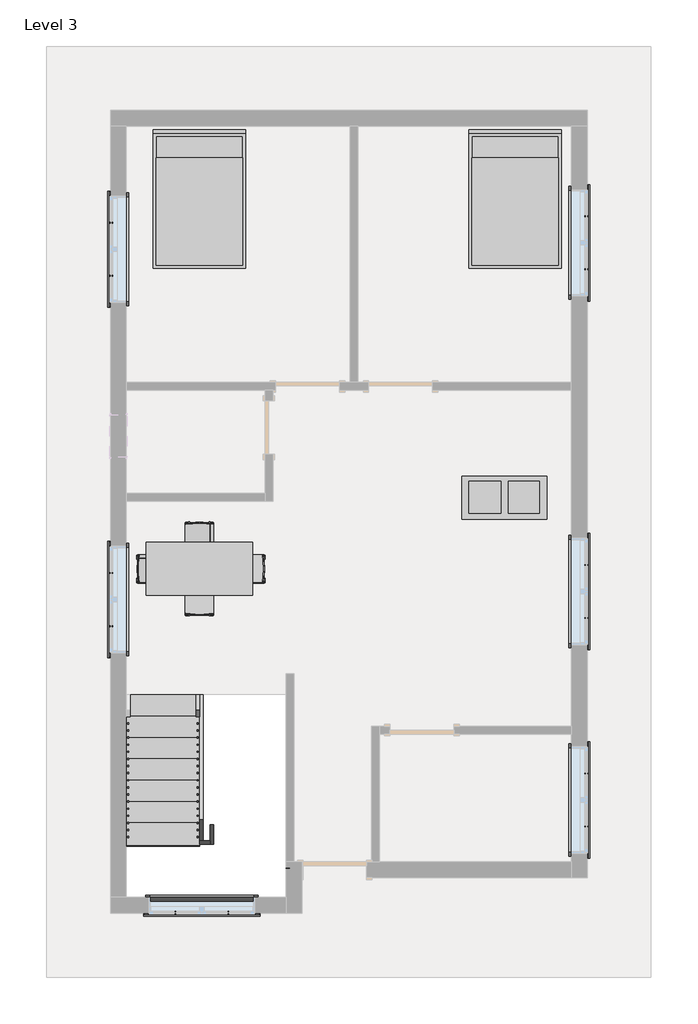
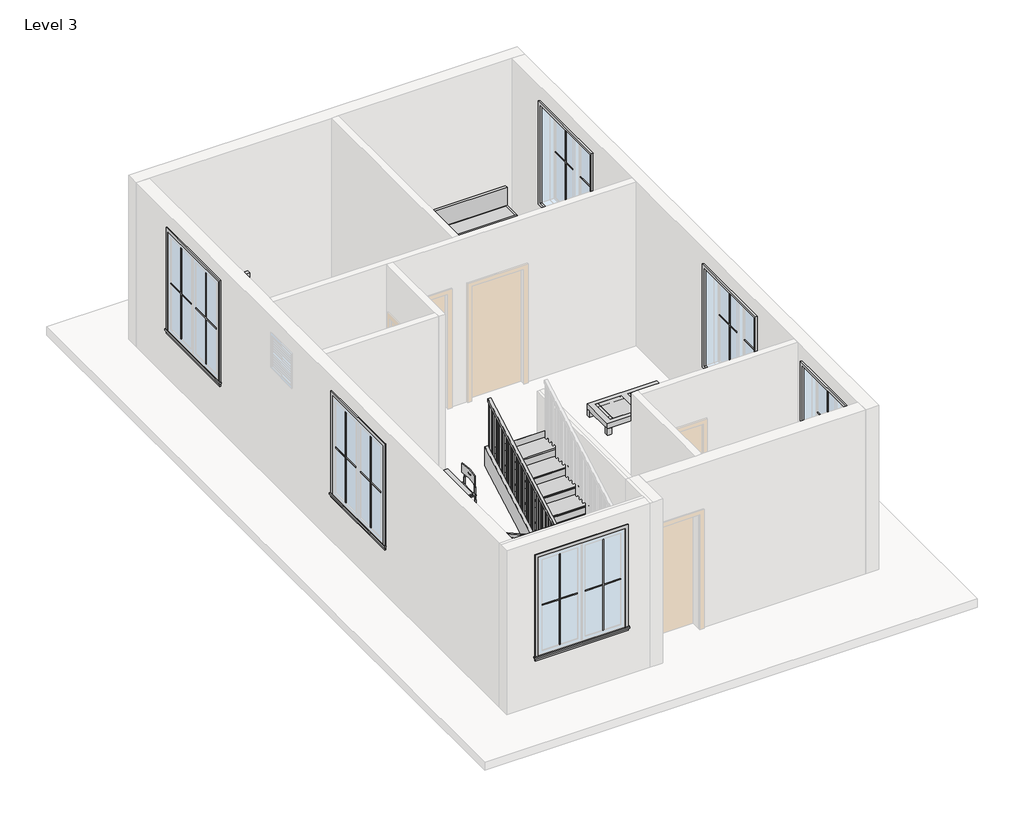
# One storey, part 3 of 3: 25 proxies, 6 members, 3 furniture elements, 1 railing, 1 stair flight.
"""IFC4 building model written with IfcOpenShell, lengths in millimetres."""

from ifc_helpers import new_model, si_unit, frame, origin, place, context, project, spatial, polyline, outline, extrude, faceted_brep, transform, mapped, element, save
from components import muntin_pattern_2x2_muntin_pattern_2x2_f6a80940, muntin_pattern_2x2_muntin_pattern_2x2_09b00a1c, trim_window_exterior_flat_with_sill_698ed857, trim_window_interior_flat_picture_frame_92551a5e, coffee_table_with_brass_mullions_11320_coffee_table_with_5962bef7, bed_17739_bed_17739_15c61121, dining_table_w_chairs_11374_0cdfc61b, stair_flight_c3010b6b

model = new_model("IFC4")

# Units and contexts
model_context = context("Model", 3, world=origin())
ifc_project = project(units=[si_unit("LENGTHUNIT", "METRE", prefix="MILLI")], contexts=[model_context])

# Site, building, storey
site = spatial("IfcSite", under=ifc_project)
building = spatial("IfcBuilding", under=site)
storey = spatial("IfcBuildingStorey", under=building, Name="Level 3", Elevation=6248.4)

# Proxies
placement = place(None, origin())
muntin_pattern_2x2_muntin_pattern_2x2_shape = muntin_pattern_2x2_muntin_pattern_2x2_f6a80940(model_context)
element("IfcBuildingElementProxy", 1, Name="Muntin Pattern_2x2 : Muntin Pattern_2x2", ObjectType="Muntin Pattern_2x2 : Muntin Pattern_2x2", at=placement, inside=storey, context=model_context, shape_type="MappedRepresentation", body=[
    mapped(muntin_pattern_2x2_muntin_pattern_2x2_shape, transform((-2773.368364, -6686.2830018, 7232.65), x_axis=(-1.0, 0.0, 0.0), y_axis=(0.0, -1.0, 0.0), z_axis=(0.0, 0.0, 1.0))),
])
element("IfcBuildingElementProxy", 2, Name="Muntin Pattern_2x2 : Muntin Pattern_2x2", ObjectType="Muntin Pattern_2x2 : Muntin Pattern_2x2", at=placement, inside=storey, context=model_context, shape_type="MappedRepresentation", body=[
    mapped(muntin_pattern_2x2_muntin_pattern_2x2_shape, transform((2349.494136, -4693.9705018, 7232.65), x_axis=(0.0, -1.0, 0.0), y_axis=(1.0, 0.0, 0.0), z_axis=(0.0, 0.0, 1.0))),
])
element("IfcBuildingElementProxy", 3, Name="Muntin Pattern_2x2 : Muntin Pattern_2x2", ObjectType="Muntin Pattern_2x2 : Muntin Pattern_2x2", at=placement, inside=storey, context=model_context, shape_type="MappedRepresentation", body=[
    mapped(muntin_pattern_2x2_muntin_pattern_2x2_shape, transform((2349.494136, -1712.6455018, 7232.65), x_axis=(0.0, -1.0, 0.0), y_axis=(1.0, 0.0, 0.0), z_axis=(0.0, 0.0, 1.0))),
])
element("IfcBuildingElementProxy", 4, Name="Muntin Pattern_2x2 : Muntin Pattern_2x2", ObjectType="Muntin Pattern_2x2 : Muntin Pattern_2x2", at=placement, inside=storey, context=model_context, shape_type="MappedRepresentation", body=[
    mapped(muntin_pattern_2x2_muntin_pattern_2x2_shape, transform((-4451.355864, -2586.5525081, 7232.65), x_axis=(0.0, 1.0, 0.0), y_axis=(-1.0, 0.0, 0.0), z_axis=(0.0, 0.0, 1.0))),
])
element("IfcBuildingElementProxy", 5, Name="Muntin Pattern_2x2 : Muntin Pattern_2x2", ObjectType="Muntin Pattern_2x2 : Muntin Pattern_2x2", at=placement, inside=storey, context=model_context, shape_type="MappedRepresentation", body=[
    mapped(muntin_pattern_2x2_muntin_pattern_2x2_shape, transform((2349.494136, 3272.1044982, 7232.65), x_axis=(0.0, -1.0, 0.0), y_axis=(1.0, 0.0, 0.0), z_axis=(0.0, 0.0, 1.0))),
])
element("IfcBuildingElementProxy", 6, Name="Muntin Pattern_2x2 : Muntin Pattern_2x2", ObjectType="Muntin Pattern_2x2 : Muntin Pattern_2x2", at=placement, inside=storey, context=model_context, shape_type="MappedRepresentation", body=[
    mapped(muntin_pattern_2x2_muntin_pattern_2x2_shape, transform((-4451.355864, 2421.2162133, 7232.65), x_axis=(0.0, 1.0, 0.0), y_axis=(-1.0, 0.0, 0.0), z_axis=(0.0, 0.0, 1.0))),
])
muntin_pattern_2x2_muntin_pattern_2x2_2_shape = muntin_pattern_2x2_muntin_pattern_2x2_09b00a1c(model_context)
element("IfcBuildingElementProxy", 7, Name="Muntin Pattern_2x2 : Muntin Pattern_2x2", ObjectType="Muntin Pattern_2x2 : Muntin Pattern_2x2", at=placement, inside=storey, context=model_context, shape_type="MappedRepresentation", body=[
    mapped(muntin_pattern_2x2_muntin_pattern_2x2_2_shape, transform((-3532.193364, -6686.2830018, 7232.65), x_axis=(1.0, 0.0, 0.0), y_axis=(0.0, 1.0, 0.0), z_axis=(0.0, 0.0, 1.0))),
])
element("IfcBuildingElementProxy", 8, Name="Muntin Pattern_2x2 : Muntin Pattern_2x2", ObjectType="Muntin Pattern_2x2 : Muntin Pattern_2x2", at=placement, inside=storey, context=model_context, shape_type="MappedRepresentation", body=[
    mapped(muntin_pattern_2x2_muntin_pattern_2x2_2_shape, transform((2349.494136, -5452.7955018, 7232.65), x_axis=(0.0, 1.0, 0.0), y_axis=(-1.0, 0.0, 0.0), z_axis=(0.0, 0.0, 1.0))),
])
element("IfcBuildingElementProxy", 9, Name="Muntin Pattern_2x2 : Muntin Pattern_2x2", ObjectType="Muntin Pattern_2x2 : Muntin Pattern_2x2", at=placement, inside=storey, context=model_context, shape_type="MappedRepresentation", body=[
    mapped(muntin_pattern_2x2_muntin_pattern_2x2_2_shape, transform((2349.494136, -2471.4705018, 7232.65), x_axis=(0.0, 1.0, 0.0), y_axis=(-1.0, 0.0, 0.0), z_axis=(0.0, 0.0, 1.0))),
])
element("IfcBuildingElementProxy", 10, Name="Muntin Pattern_2x2 : Muntin Pattern_2x2", ObjectType="Muntin Pattern_2x2 : Muntin Pattern_2x2", at=placement, inside=storey, context=model_context, shape_type="MappedRepresentation", body=[
    mapped(muntin_pattern_2x2_muntin_pattern_2x2_2_shape, transform((-4451.355864, -1827.7275081, 7232.65), x_axis=(0.0, -1.0, 0.0), y_axis=(1.0, 0.0, 0.0), z_axis=(0.0, 0.0, 1.0))),
])
element("IfcBuildingElementProxy", 11, Name="Muntin Pattern_2x2 : Muntin Pattern_2x2", ObjectType="Muntin Pattern_2x2 : Muntin Pattern_2x2", at=placement, inside=storey, context=model_context, shape_type="MappedRepresentation", body=[
    mapped(muntin_pattern_2x2_muntin_pattern_2x2_2_shape, transform((2349.494136, 2513.2794982, 7232.65), x_axis=(0.0, 1.0, 0.0), y_axis=(-1.0, 0.0, 0.0), z_axis=(0.0, 0.0, 1.0))),
])
element("IfcBuildingElementProxy", 12, Name="Muntin Pattern_2x2 : Muntin Pattern_2x2", ObjectType="Muntin Pattern_2x2 : Muntin Pattern_2x2", at=placement, inside=storey, context=model_context, shape_type="MappedRepresentation", body=[
    mapped(muntin_pattern_2x2_muntin_pattern_2x2_2_shape, transform((-4451.355864, 3180.0412133, 7232.65), x_axis=(0.0, -1.0, 0.0), y_axis=(1.0, 0.0, 0.0), z_axis=(0.0, 0.0, 1.0))),
])
trim_window_exterior_flat_with_sill_shape = trim_window_exterior_flat_with_sill_698ed857(model_context)
element("IfcBuildingElementProxy", 13, Name="Trim-Window-Exterior-Flat : with Sill", ObjectType="Trim-Window-Exterior-Flat : with Sill", at=placement, inside=storey, context=model_context, shape_type="MappedRepresentation", body=[
    mapped(trim_window_exterior_flat_with_sill_shape, transform((-3152.780864, -6695.8080018, 8991.6), x_axis=(1.0, 0.0, 0.0), y_axis=(0.0, 0.0, 1.0), z_axis=(0.0, -1.0, 0.0))),
])
element("IfcBuildingElementProxy", 14, Name="Trim-Window-Exterior-Flat : with Sill", ObjectType="Trim-Window-Exterior-Flat : with Sill", at=placement, inside=storey, context=model_context, shape_type="MappedRepresentation", body=[
    mapped(trim_window_exterior_flat_with_sill_shape, transform((2359.019136, -5073.3830018, 8991.6), x_axis=(0.0, 1.0, 0.0), y_axis=(0.0, 0.0, 1.0), z_axis=(1.0, 0.0, 0.0))),
])
element("IfcBuildingElementProxy", 15, Name="Trim-Window-Exterior-Flat : with Sill", ObjectType="Trim-Window-Exterior-Flat : with Sill", at=placement, inside=storey, context=model_context, shape_type="MappedRepresentation", body=[
    mapped(trim_window_exterior_flat_with_sill_shape, transform((2359.019136, -2092.0580018, 8991.6), x_axis=(0.0, 1.0, 0.0), y_axis=(0.0, 0.0, 1.0), z_axis=(1.0, 0.0, 0.0))),
])
element("IfcBuildingElementProxy", 16, Name="Trim-Window-Exterior-Flat : with Sill", ObjectType="Trim-Window-Exterior-Flat : with Sill", at=placement, inside=storey, context=model_context, shape_type="MappedRepresentation", body=[
    mapped(trim_window_exterior_flat_with_sill_shape, transform((-4460.880864, -2207.1400081, 8991.6), x_axis=(0.0, -1.0, 0.0), y_axis=(0.0, 0.0, 1.0), z_axis=(-1.0, 0.0, 0.0))),
])
element("IfcBuildingElementProxy", 17, Name="Trim-Window-Exterior-Flat : with Sill", ObjectType="Trim-Window-Exterior-Flat : with Sill", at=placement, inside=storey, context=model_context, shape_type="MappedRepresentation", body=[
    mapped(trim_window_exterior_flat_with_sill_shape, transform((2359.019136, 2892.6919982, 8991.6), x_axis=(0.0, 1.0, 0.0), y_axis=(0.0, 0.0, 1.0), z_axis=(1.0, 0.0, 0.0))),
])
element("IfcBuildingElementProxy", 18, Name="Trim-Window-Exterior-Flat : with Sill", ObjectType="Trim-Window-Exterior-Flat : with Sill", at=placement, inside=storey, context=model_context, shape_type="MappedRepresentation", body=[
    mapped(trim_window_exterior_flat_with_sill_shape, transform((-4460.880864, 2800.6287133, 8991.6), x_axis=(0.0, -1.0, 0.0), y_axis=(0.0, 0.0, 1.0), z_axis=(-1.0, 0.0, 0.0))),
])
trim_window_interior_flat_picture_frame_shape = trim_window_interior_flat_picture_frame_92551a5e(model_context)
element("IfcBuildingElementProxy", 19, Name="Trim-Window-Interior-Flat : Picture Frame", ObjectType="Trim-Window-Interior-Flat : Picture Frame", at=placement, inside=storey, context=model_context, shape_type="MappedRepresentation", body=[
    mapped(trim_window_interior_flat_picture_frame_shape, transform((-3152.780864, -6467.2080018, 8991.6), x_axis=(-1.0, 0.0, 0.0), y_axis=(0.0, 0.0, 1.0), z_axis=(0.0, 1.0, 0.0))),
])
element("IfcBuildingElementProxy", 20, Name="Trim-Window-Interior-Flat : Picture Frame", ObjectType="Trim-Window-Interior-Flat : Picture Frame", at=placement, inside=storey, context=model_context, shape_type="MappedRepresentation", body=[
    mapped(trim_window_interior_flat_picture_frame_shape, transform((2130.419136, -5073.3830018, 8991.6), x_axis=(0.0, -1.0, 0.0), y_axis=(0.0, 0.0, 1.0), z_axis=(-1.0, 0.0, 0.0))),
])
element("IfcBuildingElementProxy", 21, Name="Trim-Window-Interior-Flat : Picture Frame", ObjectType="Trim-Window-Interior-Flat : Picture Frame", at=placement, inside=storey, context=model_context, shape_type="MappedRepresentation", body=[
    mapped(trim_window_interior_flat_picture_frame_shape, transform((2130.419136, -2092.0580018, 8991.6), x_axis=(0.0, -1.0, 0.0), y_axis=(0.0, 0.0, 1.0), z_axis=(-1.0, 0.0, 0.0))),
])
element("IfcBuildingElementProxy", 22, Name="Trim-Window-Interior-Flat : Picture Frame", ObjectType="Trim-Window-Interior-Flat : Picture Frame", at=placement, inside=storey, context=model_context, shape_type="MappedRepresentation", body=[
    mapped(trim_window_interior_flat_picture_frame_shape, transform((-4232.280864, -2207.1400081, 8991.6), x_axis=(0.0, 1.0, 0.0), y_axis=(0.0, 0.0, 1.0), z_axis=(1.0, 0.0, 0.0))),
])
element("IfcBuildingElementProxy", 23, Name="Trim-Window-Interior-Flat : Picture Frame", ObjectType="Trim-Window-Interior-Flat : Picture Frame", at=placement, inside=storey, context=model_context, shape_type="MappedRepresentation", body=[
    mapped(trim_window_interior_flat_picture_frame_shape, transform((2130.419136, 2892.6919982, 8991.6), x_axis=(0.0, -1.0, 0.0), y_axis=(0.0, 0.0, 1.0), z_axis=(-1.0, 0.0, 0.0))),
])
element("IfcBuildingElementProxy", 24, Name="Trim-Window-Interior-Flat : Picture Frame", ObjectType="Trim-Window-Interior-Flat : Picture Frame", at=placement, inside=storey, context=model_context, shape_type="MappedRepresentation", body=[
    mapped(trim_window_interior_flat_picture_frame_shape, transform((-4232.280864, 2800.6287133, 8991.6), x_axis=(0.0, 1.0, 0.0), y_axis=(0.0, 0.0, 1.0), z_axis=(1.0, 0.0, 0.0))),
])
coffee_table_with_brass_mullions_11320_coffee_table_with_shape = coffee_table_with_brass_mullions_11320_coffee_table_with_5962bef7(model_context)
element("IfcBuildingElementProxy", 25, Name="coffee_table_with_brass_mullions_11320 : coffee_table_with_brass_mullions_11320", ObjectType="coffee_table_with_brass_mullions_11320 : coffee_table_with_brass_mullions_11320", at=placement, inside=storey, context=model_context, shape_type="MappedRepresentation", body=[
    mapped(coffee_table_with_brass_mullions_11320_coffee_table_with_shape, transform((1812.3816081, -1181.1001099, 6248.4), x_axis=(1.0, 0.0, 0.0), y_axis=(0.0, 1.0, 0.0), z_axis=(0.0, 0.0, 1.0))),
])

# Furniture
bed_17739_bed_17739_shape = bed_17739_bed_17739_15c61121(model_context)
element("IfcFurniture", 26, ObjectType="Bed_17739 : Bed_17739", at=placement, inside=storey, context=model_context, shape_type="MappedRepresentation", body=[
    mapped(bed_17739_bed_17739_shape, transform((1328.5116081, 3496.3098901, 6248.4), x_axis=(1.0, 0.0, 0.0), y_axis=(0.0, 1.0, 0.0), z_axis=(0.0, 0.0, 1.0))),
])
element("IfcFurniture", 27, ObjectType="Bed_17739 : Bed_17739", at=placement, inside=storey, context=model_context, shape_type="MappedRepresentation", body=[
    mapped(bed_17739_bed_17739_shape, transform((-3187.6083919, 3496.3098901, 6248.4), x_axis=(1.0, 0.0, 0.0), y_axis=(0.0, 1.0, 0.0), z_axis=(0.0, 0.0, 1.0))),
])
dining_table_w_chairs_11374_shape = dining_table_w_chairs_11374_0cdfc61b(model_context)
element("IfcFurniture", 28, ObjectType="Dining_Table_w_Chairs_11374", at=placement, inside=storey, context=model_context, shape_type="MappedRepresentation", body=[
    mapped(dining_table_w_chairs_11374_shape, transform((-3205.8741586, -1863.0511877, 6248.4), x_axis=(1.0, 0.0, 0.0), y_axis=(0.0, 1.0, 0.0), z_axis=(0.0, 0.0, 1.0))),
])

# Members
element("IfcMember", 29, ObjectType="Stringer - 2\" Width", at=placement, inside=storey, context=model_context, shape_type="SweptSolid", body=[
    extrude(outline(polyline([(-3571.6080018, 6455.9983948), (-3571.6080018, 6248.4), (-3825.5525046, 6248.4), (-5654.4080018, 7264.4308318), (-5654.4080018, 7613.1095059), (-3571.6080018, 6455.9983948)])), frame((-3187.6083919, 0.0, 0.0), z_axis=(1.0, 0.0, 0.0), x_axis=(0.0, 1.0, 0.0)), (0.0, 0.0, 1.0), 50.8),
])
element("IfcMember", 30, ObjectType="Stringer - 2\" Width", at=placement, inside=storey, context=model_context, shape_type="SweptSolid", body=[
    extrude(outline(polyline([(-3187.6083919, -5705.2080018), (-3187.6083919, -5654.4080018), (-3035.2083919, -5654.4080018), (-3035.2083919, -5705.2080018), (-3187.6083919, -5705.2080018)])), frame((0.0, 0.0, 7374.4666667), z_axis=(0.0, 0.0, 1.0), x_axis=(1.0, 0.0, 0.0)), (0.0, 0.0, 1.0), 304.8),
])
element("IfcMember", 31, ObjectType="Stringer - 2\" Width", at=placement, inside=storey, context=model_context, shape_type="SweptSolid", body=[
    extrude(outline(polyline([(-5705.2080018, 7374.4666667), (-5705.2080018, 7641.3317281), (-3571.6080018, 8826.6650614), (-3571.6080018, 8477.9863873), (-5557.943499, 7374.4666667), (-5705.2080018, 7374.4666667)])), frame((-3035.2083919, 0.0, 0.0), z_axis=(1.0, 0.0, 0.0), x_axis=(0.0, 1.0, 0.0)), (0.0, 0.0, 1.0), 50.8),
])
element("IfcMember", 32, ObjectType="Stringer - 2\" Width", at=placement, inside=storey, context=model_context, shape_type="SweptSolid", body=[
    extrude(outline(polyline([(-3571.6080018, 6455.9983948), (-3571.6080018, 6248.4), (-3825.5525046, 6248.4), (-6401.1125046, 7679.2666667), (-5773.4908912, 7679.2666667), (-3571.6080018, 6455.9983948)])), frame((-4283.080864, 0.0, 0.0), z_axis=(1.0, 0.0, 0.0), x_axis=(0.0, 1.0, 0.0)), (0.0, 0.0, 1.0), 50.8),
])
element("IfcMember", 33, ObjectType="Stringer - 2\" Width", at=placement, inside=storey, context=model_context, shape_type="SweptSolid", body=[
    extrude(outline(polyline([(-4283.080864, -6518.0080018), (-4283.080864, -6467.2080018), (-1946.280864, -6467.2080018), (-1946.280864, -6518.0080018), (-4283.080864, -6518.0080018)])), frame((0.0, 0.0, 7374.4666667), z_axis=(0.0, 0.0, 1.0), x_axis=(1.0, 0.0, 0.0)), (0.0, 0.0, 1.0), 304.8),
])
element("IfcMember", 34, ObjectType="Stringer - 2\" Width", at=placement, inside=storey, context=model_context, shape_type="SweptSolid", body=[
    extrude(outline(polyline([(-6185.5651124, 7374.4666667), (-3571.6080018, 8826.6650614), (-3571.6080018, 8477.9863873), (-5557.943499, 7374.4666667), (-6185.5651124, 7374.4666667)])), frame((-1946.280864, 0.0, 0.0), z_axis=(1.0, 0.0, 0.0), x_axis=(0.0, 1.0, 0.0)), (0.0, 0.0, 1.0), 50.8),
])

# Railing
element("IfcRailing", 35, ObjectType="Handrail - Rectangular", at=placement, inside=storey, context=model_context, shape_type="SolidModel", body=[
    faceted_brep([(-3187.6083919, -3571.6080018, 7332.1333333), (-3187.6083919, -3571.6080018, 7274.020221), (-3238.4083919, -3571.6080018, 7274.020221), (-3238.4083919, -3571.6080018, 7332.1333333), (-3187.6083919, -5629.0080018, 8475.1333333), (-3187.6083919, -5679.8080018, 8445.2424432), (-3238.4083919, -5679.8080018, 8445.2424432), (-3238.4083919, -5629.0080018, 8475.1333333), (-3187.6083919, -5629.0080018, 8517.4666667), (-3187.6083919, -5679.8080018, 8466.6666667), (-3238.4083919, -5679.8080018, 8466.6666667), (-3238.4083919, -5629.0080018, 8517.4666667), (-3187.6083919, -5705.2080018, 8517.4666667), (-3187.6083919, -5705.2080018, 8466.6666667), (-3238.4083919, -5756.0080018, 8466.6666667), (-3238.4083919, -5756.0080018, 8517.4666667), (-3111.4083919, -5705.2080018, 8517.4666667), (-3111.4083919, -5705.2080018, 8466.6666667), (-3111.4083919, -5756.0080018, 8466.6666667), (-3111.4083919, -5756.0080018, 8517.4666667), (-3060.6083919, -5705.2080018, 8517.4666667), (-3009.8083919, -5705.2080018, 8466.6666667), (-3009.8083919, -5756.0080018, 8466.6666667), (-3060.6083919, -5756.0080018, 8517.4666667), (-3060.6083919, -5705.2080018, 8559.8), (-3009.8083919, -5705.2080018, 8509.0), (-3009.8083919, -5756.0080018, 8509.0), (-3060.6083919, -5756.0080018, 8559.8), (-2984.4083919, -5705.2080018, 8559.8), (-2984.4083919, -5705.2080018, 8509.0), (-2933.6083919, -5756.0080018, 8509.0), (-2933.6083919, -5756.0080018, 8559.8), (-2984.4083919, -5629.0080018, 8559.8), (-2984.4083919, -5615.8443995, 8509.0), (-2933.6083919, -5615.8443995, 8509.0), (-2933.6083919, -5629.0080018, 8559.8), (-2984.4083919, -3571.6080018, 9702.8), (-2933.6083919, -3571.6080018, 9702.8), (-2933.6083919, -3571.6080018, 9644.6868876), (-2984.4083919, -3571.6080018, 9644.6868876)], [[[0, 1, 2, 3]], [[1, 0, 4, 5]], [[2, 1, 5, 6]], [[3, 2, 6, 7]], [[0, 3, 7, 4]], [[5, 4, 8, 9]], [[6, 5, 9, 10]], [[7, 6, 10, 11]], [[4, 7, 11, 8]], [[9, 8, 12, 13]], [[10, 9, 13, 14]], [[11, 10, 14, 15]], [[8, 11, 15, 12]], [[13, 12, 16, 17]], [[14, 13, 17, 18]], [[15, 14, 18, 19]], [[12, 15, 19, 16]], [[17, 16, 20, 21]], [[18, 17, 21, 22]], [[19, 18, 22, 23]], [[16, 19, 23, 20]], [[21, 20, 24, 25]], [[22, 21, 25, 26]], [[23, 22, 26, 27]], [[20, 23, 27, 24]], [[25, 24, 28, 29]], [[26, 25, 29, 30]], [[27, 26, 30, 31]], [[24, 27, 31, 28]], [[29, 28, 32, 33]], [[30, 29, 33, 34]], [[31, 30, 34, 35]], [[28, 31, 35, 32]], [[36, 37, 38, 39]], [[33, 32, 36, 39]], [[34, 33, 39, 38]], [[35, 34, 38, 37]], [[32, 35, 37, 36]]]),
    extrude(outline(polyline([(-3587.4830018, 9635.8674432), (-3587.4830018, 8619.0666667), (-3606.5330018, 8619.0666667), (-3606.5330018, 9625.2841099), (-3587.4830018, 9635.8674432)])), frame((-2968.5333919, 0.0, 0.0), z_axis=(1.0, 0.0, 0.0), x_axis=(0.0, 1.0, 0.0)), (0.0, 0.0, 1.0), 19.05),
    extrude(outline(polyline([(-3689.0830018, 9579.4229988), (-3689.0830018, 8619.0666667), (-3708.1330018, 8619.0666667), (-3708.1330018, 9568.8396654), (-3689.0830018, 9579.4229988)])), frame((-2968.5333919, 0.0, 0.0), z_axis=(1.0, 0.0, 0.0), x_axis=(0.0, 1.0, 0.0)), (0.0, 0.0, 1.0), 19.05),
    extrude(outline(polyline([(-3790.6830018, 9522.9785543), (-3790.6830018, 8619.0666667), (-3809.7330018, 8619.0666667), (-3809.7330018, 9512.395221), (-3790.6830018, 9522.9785543)])), frame((-2968.5333919, 0.0, 0.0), z_axis=(1.0, 0.0, 0.0), x_axis=(0.0, 1.0, 0.0)), (0.0, 0.0, 1.0), 19.05),
    extrude(outline(polyline([(-3892.2830018, 9466.5341099), (-3892.2830018, 8449.7333333), (-3911.3330018, 8449.7333333), (-3911.3330018, 9455.9507765), (-3892.2830018, 9466.5341099)])), frame((-2968.5333919, 0.0, 0.0), z_axis=(1.0, 0.0, 0.0), x_axis=(0.0, 1.0, 0.0)), (0.0, 0.0, 1.0), 19.05),
    extrude(outline(polyline([(-3993.8830018, 9410.0896654), (-3993.8830018, 8449.7333333), (-4012.9330018, 8449.7333333), (-4012.9330018, 9399.5063321), (-3993.8830018, 9410.0896654)])), frame((-2968.5333919, 0.0, 0.0), z_axis=(1.0, 0.0, 0.0), x_axis=(0.0, 1.0, 0.0)), (0.0, 0.0, 1.0), 19.05),
    extrude(outline(polyline([(-4095.4830018, 9353.645221), (-4095.4830018, 8449.7333333), (-4114.5330018, 8449.7333333), (-4114.5330018, 9343.0618876), (-4095.4830018, 9353.645221)])), frame((-2968.5333919, 0.0, 0.0), z_axis=(1.0, 0.0, 0.0), x_axis=(0.0, 1.0, 0.0)), (0.0, 0.0, 1.0), 19.05),
    extrude(outline(polyline([(-4197.0830018, 9297.2007765), (-4197.0830018, 8280.4), (-4216.1330018, 8280.4), (-4216.1330018, 9286.6174432), (-4197.0830018, 9297.2007765)])), frame((-2968.5333919, 0.0, 0.0), z_axis=(1.0, 0.0, 0.0), x_axis=(0.0, 1.0, 0.0)), (0.0, 0.0, 1.0), 19.05),
    extrude(outline(polyline([(-4298.6830018, 9240.7563321), (-4298.6830018, 8280.4), (-4317.7330018, 8280.4), (-4317.7330018, 9230.1729988), (-4298.6830018, 9240.7563321)])), frame((-2968.5333919, 0.0, 0.0), z_axis=(1.0, 0.0, 0.0), x_axis=(0.0, 1.0, 0.0)), (0.0, 0.0, 1.0), 19.05),
    extrude(outline(polyline([(-4400.2830018, 9184.3118876), (-4400.2830018, 8280.4), (-4419.3330018, 8280.4), (-4419.3330018, 9173.7285543), (-4400.2830018, 9184.3118876)])), frame((-2968.5333919, 0.0, 0.0), z_axis=(1.0, 0.0, 0.0), x_axis=(0.0, 1.0, 0.0)), (0.0, 0.0, 1.0), 19.05),
    extrude(outline(polyline([(-4501.8830018, 9127.8674432), (-4501.8830018, 8111.0666667), (-4520.9330018, 8111.0666667), (-4520.9330018, 9117.2841099), (-4501.8830018, 9127.8674432)])), frame((-2968.5333919, 0.0, 0.0), z_axis=(1.0, 0.0, 0.0), x_axis=(0.0, 1.0, 0.0)), (0.0, 0.0, 1.0), 19.05),
    extrude(outline(polyline([(-4603.4830018, 9071.4229988), (-4603.4830018, 8111.0666667), (-4622.5330018, 8111.0666667), (-4622.5330018, 9060.8396654), (-4603.4830018, 9071.4229988)])), frame((-2968.5333919, 0.0, 0.0), z_axis=(1.0, 0.0, 0.0), x_axis=(0.0, 1.0, 0.0)), (0.0, 0.0, 1.0), 19.05),
    extrude(outline(polyline([(-4705.0830018, 9014.9785543), (-4705.0830018, 8111.0666667), (-4724.1330018, 8111.0666667), (-4724.1330018, 9004.395221), (-4705.0830018, 9014.9785543)])), frame((-2968.5333919, 0.0, 0.0), z_axis=(1.0, 0.0, 0.0), x_axis=(0.0, 1.0, 0.0)), (0.0, 0.0, 1.0), 19.05),
    extrude(outline(polyline([(-4806.6830018, 8958.5341099), (-4806.6830018, 7941.7333333), (-4825.7330018, 7941.7333333), (-4825.7330018, 8947.9507765), (-4806.6830018, 8958.5341099)])), frame((-2968.5333919, 0.0, 0.0), z_axis=(1.0, 0.0, 0.0), x_axis=(0.0, 1.0, 0.0)), (0.0, 0.0, 1.0), 19.05),
    extrude(outline(polyline([(-4908.2830018, 8902.0896654), (-4908.2830018, 7941.7333333), (-4927.3330018, 7941.7333333), (-4927.3330018, 8891.5063321), (-4908.2830018, 8902.0896654)])), frame((-2968.5333919, 0.0, 0.0), z_axis=(1.0, 0.0, 0.0), x_axis=(0.0, 1.0, 0.0)), (0.0, 0.0, 1.0), 19.05),
    extrude(outline(polyline([(-5009.8830018, 8845.645221), (-5009.8830018, 7941.7333333), (-5028.9330018, 7941.7333333), (-5028.9330018, 8835.0618876), (-5009.8830018, 8845.645221)])), frame((-2968.5333919, 0.0, 0.0), z_axis=(1.0, 0.0, 0.0), x_axis=(0.0, 1.0, 0.0)), (0.0, 0.0, 1.0), 19.05),
    extrude(outline(polyline([(-5111.4830018, 8789.2007765), (-5111.4830018, 7772.4), (-5130.5330018, 7772.4), (-5130.5330018, 8778.6174432), (-5111.4830018, 8789.2007765)])), frame((-2968.5333919, 0.0, 0.0), z_axis=(1.0, 0.0, 0.0), x_axis=(0.0, 1.0, 0.0)), (0.0, 0.0, 1.0), 19.05),
    extrude(outline(polyline([(-5213.0830018, 8732.7563321), (-5213.0830018, 7772.4), (-5232.1330018, 7772.4), (-5232.1330018, 8722.1729988), (-5213.0830018, 8732.7563321)])), frame((-2968.5333919, 0.0, 0.0), z_axis=(1.0, 0.0, 0.0), x_axis=(0.0, 1.0, 0.0)), (0.0, 0.0, 1.0), 19.05),
    extrude(outline(polyline([(-5314.6830018, 8676.3118876), (-5314.6830018, 7772.4), (-5333.7330018, 7772.4), (-5333.7330018, 8665.7285543), (-5314.6830018, 8676.3118876)])), frame((-2968.5333919, 0.0, 0.0), z_axis=(1.0, 0.0, 0.0), x_axis=(0.0, 1.0, 0.0)), (0.0, 0.0, 1.0), 19.05),
    extrude(outline(polyline([(-5416.2830018, 8619.8674432), (-5416.2830018, 7603.0666667), (-5435.3330018, 7603.0666667), (-5435.3330018, 8609.2841099), (-5416.2830018, 8619.8674432)])), frame((-2968.5333919, 0.0, 0.0), z_axis=(1.0, 0.0, 0.0), x_axis=(0.0, 1.0, 0.0)), (0.0, 0.0, 1.0), 19.05),
    extrude(outline(polyline([(-5517.8830018, 8563.4229988), (-5517.8830018, 7603.0666667), (-5536.9330018, 7603.0666667), (-5536.9330018, 8552.8396654), (-5517.8830018, 8563.4229988)])), frame((-2968.5333919, 0.0, 0.0), z_axis=(1.0, 0.0, 0.0), x_axis=(0.0, 1.0, 0.0)), (0.0, 0.0, 1.0), 19.05),
    extrude(outline(polyline([(-5619.4830018, 8506.9785543), (-5619.4830018, 7603.0666667), (-5638.5330018, 7603.0666667), (-5638.5330018, 8496.395221), (-5619.4830018, 8506.9785543)])), frame((-2968.5333919, 0.0, 0.0), z_axis=(1.0, 0.0, 0.0), x_axis=(0.0, 1.0, 0.0)), (0.0, 0.0, 1.0), 19.05),
    extrude(outline(polyline([(-3019.3333919, -5721.0830018), (-3000.2833919, -5721.0830018), (-3000.2833919, -5740.1330018), (-3019.3333919, -5740.1330018), (-3019.3333919, -5721.0830018)])), frame((0.0, 0.0, 7603.0666667), z_axis=(0.0, 0.0, 1.0), x_axis=(1.0, 0.0, 0.0)), (0.0, 0.0, 1.0), 905.9333333),
    extrude(outline(polyline([(-3120.9333919, -5721.0830018), (-3101.8833919, -5721.0830018), (-3101.8833919, -5740.1330018), (-3120.9333919, -5740.1330018), (-3120.9333919, -5721.0830018)])), frame((0.0, 0.0, 7603.0666667), z_axis=(0.0, 0.0, 1.0), x_axis=(1.0, 0.0, 0.0)), (0.0, 0.0, 1.0), 863.6),
    extrude(outline(polyline([(-3203.4833919, -5695.6830018), (-3203.4833919, -5714.7330018), (-3222.5333919, -5714.7330018), (-3222.5333919, -5695.6830018), (-3203.4833919, -5695.6830018)])), frame((0.0, 0.0, 7603.0666667), z_axis=(0.0, 0.0, 1.0), x_axis=(1.0, 0.0, 0.0)), (0.0, 0.0, 1.0), 863.6),
    extrude(outline(polyline([(-5594.0830018, 8397.6174432), (-5594.0830018, 7433.7333333), (-5613.1330018, 7433.7333333), (-5613.1330018, 8408.2007765), (-5594.0830018, 8397.6174432)])), frame((-3222.5333919, 0.0, 0.0), z_axis=(1.0, 0.0, 0.0), x_axis=(0.0, 1.0, 0.0)), (0.0, 0.0, 1.0), 19.05),
    extrude(outline(polyline([(-5492.4830018, 8341.1729988), (-5492.4830018, 7433.7333333), (-5511.5330018, 7433.7333333), (-5511.5330018, 8351.7563321), (-5492.4830018, 8341.1729988)])), frame((-3222.5333919, 0.0, 0.0), z_axis=(1.0, 0.0, 0.0), x_axis=(0.0, 1.0, 0.0)), (0.0, 0.0, 1.0), 19.05),
    extrude(outline(polyline([(-5390.8830018, 8284.7285543), (-5390.8830018, 7433.7333333), (-5409.9330018, 7433.7333333), (-5409.9330018, 8295.3118876), (-5390.8830018, 8284.7285543)])), frame((-3222.5333919, 0.0, 0.0), z_axis=(1.0, 0.0, 0.0), x_axis=(0.0, 1.0, 0.0)), (0.0, 0.0, 1.0), 19.05),
    extrude(outline(polyline([(-5289.2830018, 8228.2841099), (-5289.2830018, 7264.4), (-5308.3330018, 7264.4), (-5308.3330018, 8238.8674432), (-5289.2830018, 8228.2841099)])), frame((-3222.5333919, 0.0, 0.0), z_axis=(1.0, 0.0, 0.0), x_axis=(0.0, 1.0, 0.0)), (0.0, 0.0, 1.0), 19.05),
    extrude(outline(polyline([(-5187.6830018, 8171.8396654), (-5187.6830018, 7264.4), (-5206.7330018, 7264.4), (-5206.7330018, 8182.4229988), (-5187.6830018, 8171.8396654)])), frame((-3222.5333919, 0.0, 0.0), z_axis=(1.0, 0.0, 0.0), x_axis=(0.0, 1.0, 0.0)), (0.0, 0.0, 1.0), 19.05),
    extrude(outline(polyline([(-5086.0830018, 8115.395221), (-5086.0830018, 7264.4), (-5105.1330018, 7264.4), (-5105.1330018, 8125.9785543), (-5086.0830018, 8115.395221)])), frame((-3222.5333919, 0.0, 0.0), z_axis=(1.0, 0.0, 0.0), x_axis=(0.0, 1.0, 0.0)), (0.0, 0.0, 1.0), 19.05),
    extrude(outline(polyline([(-4984.4830018, 8058.9507765), (-4984.4830018, 7095.0666667), (-5003.5330018, 7095.0666667), (-5003.5330018, 8069.5341099), (-4984.4830018, 8058.9507765)])), frame((-3222.5333919, 0.0, 0.0), z_axis=(1.0, 0.0, 0.0), x_axis=(0.0, 1.0, 0.0)), (0.0, 0.0, 1.0), 19.05),
    extrude(outline(polyline([(-4882.8830018, 8002.5063321), (-4882.8830018, 7095.0666667), (-4901.9330018, 7095.0666667), (-4901.9330018, 8013.0896654), (-4882.8830018, 8002.5063321)])), frame((-3222.5333919, 0.0, 0.0), z_axis=(1.0, 0.0, 0.0), x_axis=(0.0, 1.0, 0.0)), (0.0, 0.0, 1.0), 19.05),
    extrude(outline(polyline([(-4781.2830018, 7946.0618876), (-4781.2830018, 7095.0666667), (-4800.3330018, 7095.0666667), (-4800.3330018, 7956.645221), (-4781.2830018, 7946.0618876)])), frame((-3222.5333919, 0.0, 0.0), z_axis=(1.0, 0.0, 0.0), x_axis=(0.0, 1.0, 0.0)), (0.0, 0.0, 1.0), 19.05),
    extrude(outline(polyline([(-4679.6830018, 7889.6174432), (-4679.6830018, 6925.7333333), (-4698.7330018, 6925.7333333), (-4698.7330018, 7900.2007765), (-4679.6830018, 7889.6174432)])), frame((-3222.5333919, 0.0, 0.0), z_axis=(1.0, 0.0, 0.0), x_axis=(0.0, 1.0, 0.0)), (0.0, 0.0, 1.0), 19.05),
    extrude(outline(polyline([(-4578.0830018, 7833.1729988), (-4578.0830018, 6925.7333333), (-4597.1330018, 6925.7333333), (-4597.1330018, 7843.7563321), (-4578.0830018, 7833.1729988)])), frame((-3222.5333919, 0.0, 0.0), z_axis=(1.0, 0.0, 0.0), x_axis=(0.0, 1.0, 0.0)), (0.0, 0.0, 1.0), 19.05),
    extrude(outline(polyline([(-4476.4830018, 7776.7285543), (-4476.4830018, 6925.7333333), (-4495.5330018, 6925.7333333), (-4495.5330018, 7787.3118876), (-4476.4830018, 7776.7285543)])), frame((-3222.5333919, 0.0, 0.0), z_axis=(1.0, 0.0, 0.0), x_axis=(0.0, 1.0, 0.0)), (0.0, 0.0, 1.0), 19.05),
    extrude(outline(polyline([(-4374.8830018, 7720.2841099), (-4374.8830018, 6756.4), (-4393.9330018, 6756.4), (-4393.9330018, 7730.8674432), (-4374.8830018, 7720.2841099)])), frame((-3222.5333919, 0.0, 0.0), z_axis=(1.0, 0.0, 0.0), x_axis=(0.0, 1.0, 0.0)), (0.0, 0.0, 1.0), 19.05),
    extrude(outline(polyline([(-4273.2830018, 7663.8396654), (-4273.2830018, 6756.4), (-4292.3330018, 6756.4), (-4292.3330018, 7674.4229988), (-4273.2830018, 7663.8396654)])), frame((-3222.5333919, 0.0, 0.0), z_axis=(1.0, 0.0, 0.0), x_axis=(0.0, 1.0, 0.0)), (0.0, 0.0, 1.0), 19.05),
    extrude(outline(polyline([(-4171.6830018, 7607.395221), (-4171.6830018, 6756.4), (-4190.7330018, 6756.4), (-4190.7330018, 7617.9785543), (-4171.6830018, 7607.395221)])), frame((-3222.5333919, 0.0, 0.0), z_axis=(1.0, 0.0, 0.0), x_axis=(0.0, 1.0, 0.0)), (0.0, 0.0, 1.0), 19.05),
    extrude(outline(polyline([(-4070.0830018, 7550.9507765), (-4070.0830018, 6587.0666667), (-4089.1330018, 6587.0666667), (-4089.1330018, 7561.5341099), (-4070.0830018, 7550.9507765)])), frame((-3222.5333919, 0.0, 0.0), z_axis=(1.0, 0.0, 0.0), x_axis=(0.0, 1.0, 0.0)), (0.0, 0.0, 1.0), 19.05),
    extrude(outline(polyline([(-3968.4830018, 7494.5063321), (-3968.4830018, 6587.0666667), (-3987.5330018, 6587.0666667), (-3987.5330018, 7505.0896654), (-3968.4830018, 7494.5063321)])), frame((-3222.5333919, 0.0, 0.0), z_axis=(1.0, 0.0, 0.0), x_axis=(0.0, 1.0, 0.0)), (0.0, 0.0, 1.0), 19.05),
    extrude(outline(polyline([(-3866.8830018, 7438.0618876), (-3866.8830018, 6587.0666667), (-3885.9330018, 6587.0666667), (-3885.9330018, 7448.645221), (-3866.8830018, 7438.0618876)])), frame((-3222.5333919, 0.0, 0.0), z_axis=(1.0, 0.0, 0.0), x_axis=(0.0, 1.0, 0.0)), (0.0, 0.0, 1.0), 19.05),
    extrude(outline(polyline([(-3765.2830018, 7381.6174432), (-3765.2830018, 6417.7333333), (-3784.3330018, 6417.7333333), (-3784.3330018, 7392.2007765), (-3765.2830018, 7381.6174432)])), frame((-3222.5333919, 0.0, 0.0), z_axis=(1.0, 0.0, 0.0), x_axis=(0.0, 1.0, 0.0)), (0.0, 0.0, 1.0), 19.05),
    extrude(outline(polyline([(-3663.6830018, 7325.1729988), (-3663.6830018, 6417.7333333), (-3682.7330018, 6417.7333333), (-3682.7330018, 7335.7563321), (-3663.6830018, 7325.1729988)])), frame((-3222.5333919, 0.0, 0.0), z_axis=(1.0, 0.0, 0.0), x_axis=(0.0, 1.0, 0.0)), (0.0, 0.0, 1.0), 19.05),
    extrude(outline(polyline([(-2968.5333919, -5721.0830018), (-2949.4833919, -5721.0830018), (-2949.4833919, -5740.1330018), (-2968.5333919, -5740.1330018), (-2968.5333919, -5721.0830018)])), frame((0.0, 0.0, 7603.0666667), z_axis=(0.0, 0.0, 1.0), x_axis=(1.0, 0.0, 0.0)), (0.0, 0.0, 1.0), 905.9333333),
    extrude(outline(polyline([(-3203.4833919, -5721.0830018), (-3203.4833919, -5740.1330018), (-3222.5333919, -5740.1330018), (-3222.5333919, -5721.0830018), (-3203.4833919, -5721.0830018)])), frame((0.0, 0.0, 7603.0666667), z_axis=(0.0, 0.0, 1.0), x_axis=(1.0, 0.0, 0.0)), (0.0, 0.0, 1.0), 863.6),
    extrude(outline(polyline([(-3571.6080018, 9644.6868876), (-3571.6080018, 8619.0666667), (-3590.6580018, 8619.0666667), (-3590.6580018, 9634.1035543), (-3571.6080018, 9644.6868876)])), frame((-2968.5333919, 0.0, 0.0), z_axis=(1.0, 0.0, 0.0), x_axis=(0.0, 1.0, 0.0)), (0.0, 0.0, 1.0), 19.05),
    extrude(outline(polyline([(-3571.6080018, 7274.020221), (-3571.6080018, 6417.7333333), (-3590.6580018, 6417.7333333), (-3590.6580018, 7284.6035543), (-3571.6080018, 7274.020221)])), frame((-3222.5333919, 0.0, 0.0), z_axis=(1.0, 0.0, 0.0), x_axis=(0.0, 1.0, 0.0)), (0.0, 0.0, 1.0), 19.05),
])

# Stair flight
stair_flight_shape = stair_flight_c3010b6b(model_context)
element("IfcStairFlight", 36, ObjectType="2\" Tread 1\" Nosing 1/4\" Riser", at=placement, inside=storey, context=model_context, shape_type="MappedRepresentation", body=[
    mapped(stair_flight_shape, transform((0.0, 0.0, 0.0), x_axis=(1.0, 0.0, 0.0), y_axis=(0.0, 1.0, 0.0), z_axis=(0.0, 0.0, 1.0))),
])

save(model, "model.ifc")

# Revit data of these elements
# Type "Muntin Pattern_2x2 : Muntin Pattern_2x2"
#   Width [instance default] = 4' - 0"
#   Thickness = 0' - 0 1/2"
#   Height [instance default] = 4' - 0"
#   Distance = 0' - 0 3/4"
#   Interior Material [instance default] = none
#   Exterior Material [instance default] = none
#   Default Elevation = 0
# Type "Trim-Window-Exterior-Flat : with Sill"
#   Trim Width = 0' - 2 1/4"
#   Trim Thickness_Picture Frame = 0' - 1 1/4"
#   Trim Thickness_with Sill = 0' - 0 3/4"
#   Sill Thickness = 0' - 1 1/4"
#   Opening Width [instance default] = 2' - 0"
#   Opening Height [instance default] = 3' - 0"
#   Default Elevation = 4' - 0"
#   Sill = yes
#   Picture Frame = no
#   Trim Material [instance default] = none
# Type "Trim-Window-Interior-Flat : Picture Frame"
#   Trim Thickness_Picture Frame = 0' - 1 1/4"
#   Trim Width = 0' - 2 1/4"
#   Trim Thickness_with Sill = 0' - 0 3/4"
#   Sill Thickness = 0' - 1 1/4"
#   Opening Width [instance default] = 2' - 0"
#   Opening Height [instance default] = 3' - 0"
#   Default Elevation = 4' - 0"
#   Sill = no
#   Picture Frame = yes
#   Trim Material [instance default] = none
# Type "coffee_table_with_brass_mullions_11320 : coffee_table_with_brass_mullions_11320"
#   Default Elevation = 0
# Type "Bed_17739 : Bed_17739"
#   Default Elevation = 0
# Type "Dining_Table_w_Chairs_11374"
#   Default Elevation = 0
#   Assembly Code = ""
# Type "Handrail - Rectangular"
#   Assembly Code = "C2010400"
#   built-in parameter 1008612 = 0.0416667 (stored number, unit not read)
#   built-in parameter 1008611 = 0.0416667 (stored number, unit not read)
#   built-in parameter 1008609 = 0.333333 (stored number, unit not read)
#   built-in parameter 1008604 = 0.166667 (stored number, unit not read)
#   built-in parameter 1008603 = 0.166667 (stored number, unit not read)
#   Railing Height = 3' - 0"
#   built-in parameter 1008630 = 2
#   built-in parameter 1008610 = 2
#   built-in parameter 1008618 = Baluster - Square : 3/4"
# Elements 1, 2, 3, 4, 5, 6, 7, 8, 9, 10, 11, 12 (IfcBuildingElementProxy, "Muntin Pattern_2x2 : Muntin Pattern_2x2")
#   Width = 2' - 0 5/8"
#   Height = 5' - 6 1/2"
#   Interior Material = Wood - Stained
#   Exterior Material = Clad - White
#   Phase Created = New Construction
#   Materials on its faces: "Clad - White", "Wood - Stained"
# Elements 13, 14, 15, 16, 17, 18 (IfcBuildingElementProxy, "Trim-Window-Exterior-Flat : with Sill")
#   Opening Width = 5' - 0"
#   Opening Height = 6' - 0"
#   Trim Material = Clad - White
#   Phase Created = New Construction
#   Materials on its faces: "Clad - White"
# Elements 19, 20, 21, 22, 23, 24 (IfcBuildingElementProxy, "Trim-Window-Interior-Flat : Picture Frame")
#   Opening Width = 5' - 0"
#   Opening Height = 6' - 0"
#   Trim Material = Wood - Stained
#   Phase Created = New Construction
#   Materials on its faces: "Wood - Stained"
# Element 25 (IfcBuildingElementProxy, "coffee_table_with_brass_mullions_11320 : coffee_table_with_brass_mullions_11320")
#   Phase Created = New Construction
#   Materials on its faces: "Default Wall", "TABLE", "Glass", "Default"
# Elements 26, 27 (IfcFurniture, "Bed_17739 : Bed_17739")
#   Phase Created = New Construction
#   Materials on its faces: "legs", "sheets", "bed frame", "Blanket"
# Element 28 (IfcFurniture, "Dining_Table_w_Chairs_11374")
#   Phase Created = New Construction
# Elements 29, 30, 31, 32, 33, 34 (IfcMember, "Stringer - 2\" Width")
#   Phase Created = New Construction
# Element 35 (IfcRailing, "Handrail - Rectangular")
#   Phase Created = New Construction
# Element 36 (IfcStairFlight, "2\" Tread 1\" Nosing 1/4\" Riser")
#   Phase Created = New Construction
# Materials
#   "Clad - White": class "Wood", colour RGB 242 242 238, transparency 0, Cost = 0
#   "Wood - Stained": class "Wood", colour RGB 224 178 126, transparency 0, Cost = 0
#   "Default Wall": colour RGB 128 128 128, transparency 0, Cost = 0
#   "TABLE": class "Generic", colour RGB 120 120 120, transparency 0, Cost = 0
#   "Glass": class "Glass", colour RGB 0 128 192, transparency 0.75, Description = "Soda Lime Glass", Cost = 0
#   "Default": colour RGB 127 127 127, transparency 0, Cost = 0
#   "legs": colour RGB 90 73 37, transparency 0, Cost = 0
#   "sheets": colour RGB 200 195 176, transparency 0, Cost = 0
#   "bed frame": colour RGB 90 73 37, transparency 0, Cost = 0
#   "Blanket": class "System", colour RGB 59 0 1, transparency 0, Cost = 0
